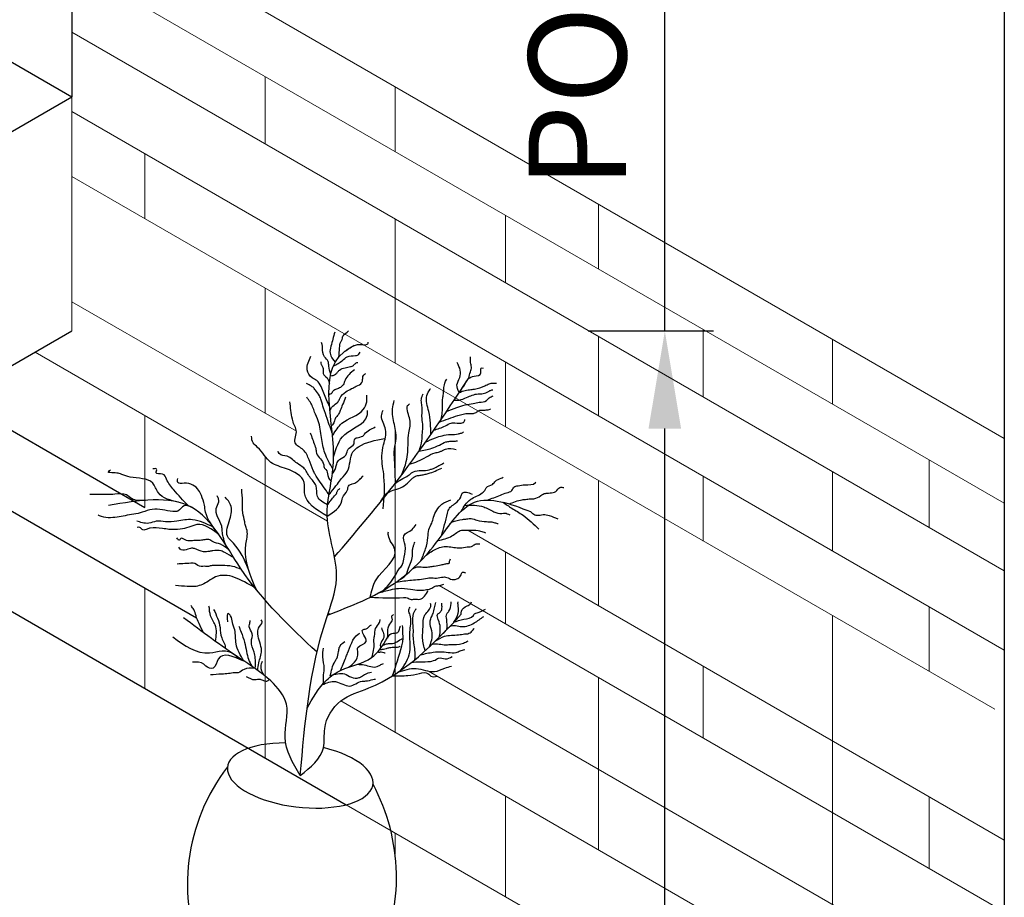
# Model space of a CAD drawing. Units: inches. Extents: x 5770 to 11891, y 3254 to 6808.
# Tile 10 of 15: x 6048 to 6073, y 3414 to 3436. Entities that reach past the tile are written whole.
import ezdxf

# ---------------------------------------------------------------- set-up
doc = ezdxf.new("R2010")
doc.units = ezdxf.units.IN
for name, color, linetype, lineweight in [('A-ANNO-DIMS', 2, 'Continuous', 18), ('A-DOOR', 4, 'Continuous', 25), ('A-FURN', 8, 'Continuous', 25), ('A-GLAZ', 4, 'Continuous', 25), ('A-WALL-PATT', 8, 'Continuous', 13)]:
    doc.layers.add(name, color=color, linetype=linetype, lineweight=lineweight)
doc.styles.get("Standard").update_dxf_attribs({"font": 'arial.ttf'})
doc.dimstyles.new('ISO-25', dxfattribs={"dimtxt": 2.5, "dimasz": 2.5, "dimexe": 1.25, "dimexo": 0.625, "dimtad": 1, "dimdec": 0, "dimlunit": 3, "dimtxsty": 'Standard', "dimcen": 2.5, "dimadec": 0, "dimazin": 0, "dimtfac": 1, "dimtdec": 0, "dimtmove": 0, "dimatfit": 3, "dimfxl": 1, "dimarcsym": 0})

# ---------------------------------------------------------------- blocks, each defined once
blk = doc.blocks.new('POT TREE')
for centre, radius, start, end in [((6057.241, 3414.341), 4.914, 142.3065, 203.4115), ((6052.61, 3414.509), 5.072, 334.4796, 28.1737), ((6055.12, 3416.4), 3.962, 226.5306, 307.3215), ((6054.997, 3414.987), 3.448, 228.9077, 309.4208)]:
    blk.add_arc(centre, radius, start, end)
blk.add_ellipse((6055.216, 3417.125), major_axis=(-1.864, 0.221), ratio=0.431649, start_param=4.964377, end_param=10.722247)
for points, knots in [([(6056.099, 3428.486), (6056.067, 3428.368), (6056.02, 3428.192), (6055.948, 3427.91), (6056.053, 3427.786), (6056.115, 3427.713)], [0, 0, 0, 0, 0.3734405, 0.5554394, 0.8239698, 0.8239698, 0.8239698, 0.8239698]), ([(6056.207, 3427.847), (6056.213, 3427.924), (6056.224, 3428.053), (6056.232, 3428.215), (6056.298, 3428.293), (6056.297, 3428.355), (6056.343, 3428.437), (6056.403, 3428.481), (6056.451, 3428.516)], [0, 0, 0, 0, 0.2339594, 0.3926456, 0.4649395, 0.5251746, 0.5691994, 0.7434006, 0.7434006, 0.7434006, 0.7434006]), ([(6055.216, 3417.125), (6055.336, 3418.48), (6055.487, 3420.181), (6056.331, 3422.342), (6055.715, 3423.715), (6056.354, 3425.55), (6055.582, 3427.539), (6056.504, 3428.093), (6056.597, 3428.149)], [0, 0, 0, 0, 4.080433, 5.124412, 6.755782, 8.14589, 10.974647, 11.292118, 11.292118, 11.292118, 11.292118]), ([(6056, 3427.411), (6055.979, 3427.477), (6055.946, 3427.582), (6055.946, 3427.752), (6055.806, 3427.869), (6055.784, 3428.034), (6055.784, 3428.159), (6055.766, 3428.202), (6055.759, 3428.218)], [0, 0, 0, 0, 0.2083526, 0.33199, 0.4828354, 0.7148467, 0.8018251, 0.8541407, 0.8541407, 0.8541407, 0.8541407]), ([(6056.371, 3428.002), (6056.422, 3428.039), (6056.532, 3428.118), (6056.727, 3428.199), (6056.886, 3428.139), (6056.964, 3428.199), (6056.961, 3428.223), (6056.96, 3428.232)], [0, 0, 0, 0, 0.1895566, 0.4093046, 0.6024508, 0.6414497, 0.6690189, 0.6690189, 0.6690189, 0.6690189]), ([(6055.967, 3426.585), (6055.915, 3426.698), (6055.838, 3426.866), (6055.755, 3427.096), (6055.662, 3427.248), (6055.479, 3427.316), (6055.344, 3427.566), (6055.436, 3427.759), (6055.492, 3427.874)], [0, 0, 0, 0, 0.371816, 0.552306, 0.74044, 0.877889, 1.120726, 1.482251, 1.482251, 1.482251, 1.482251]), ([(6056.064, 3427.611), (6056.145, 3427.655), (6056.269, 3427.724), (6056.427, 3427.889), (6056.588, 3427.869), (6056.72, 3427.903), (6056.741, 3427.953), (6056.749, 3427.972)], [0, 0, 0, 0, 0.2777951, 0.4294687, 0.6442569, 0.739735, 0.8005553, 0.8005553, 0.8005553, 0.8005553]), ([(6059.539, 3427.305), (6059.549, 3427.361), (6059.566, 3427.456), (6059.622, 3427.589), (6059.57, 3427.693), (6059.584, 3427.781), (6059.582, 3427.83), (6059.582, 3427.851)], [0, 0, 0, 0, 0.170284, 0.2915753, 0.4095788, 0.4920381, 0.5552227, 0.5552227, 0.5552227, 0.5552227]), ([(6055.746, 3427.727), (6055.745, 3427.704), (6055.742, 3427.656), (6055.802, 3427.595), (6055.813, 3427.51), (6055.793, 3427.397), (6055.923, 3427.324), (6055.949, 3427.228), (6055.963, 3427.179)], [0, 0, 0, 0, 0.0663677, 0.1385674, 0.2396579, 0.315315, 0.459478, 0.6088633, 0.6088633, 0.6088633, 0.6088633]), ([(6055.99, 3427.367), (6056.038, 3427.373), (6056.112, 3427.383), (6056.172, 3427.461), (6056.237, 3427.541), (6056.366, 3427.57), (6056.481, 3427.602), (6056.575, 3427.618), (6056.602, 3427.667), (6056.64, 3427.68), (6056.661, 3427.712), (6056.683, 3427.71), (6056.69, 3427.709)], [0, 0, 0, 0, 0.1365482, 0.2128619, 0.286554, 0.4402885, 0.5819688, 0.663825, 0.70336, 0.7384662, 0.7808805, 0.8013382, 0.8013382, 0.8013382, 0.8013382]), ([(6059.29, 3426.939), (6059.259, 3427.006), (6059.196, 3427.136), (6059.318, 3427.315), (6059.332, 3427.522), (6059.269, 3427.641), (6059.235, 3427.705)], [0, 0, 0, 0, 0.2050478, 0.4040971, 0.5914015, 0.8021175, 0.8021175, 0.8021175, 0.8021175]), ([(6059.29, 3426.939), (6059.343, 3427.011), (6059.426, 3427.125), (6059.515, 3427.313), (6059.674, 3427.364), (6059.891, 3427.379), (6059.816, 3427.58), (6059.884, 3427.567), (6059.904, 3427.563)], [0, 0, 0, 0, 0.2714027, 0.4305119, 0.5814667, 0.7785807, 0.9004742, 0.951926, 0.951926, 0.951926, 0.951926]), ([(6056.605, 3427.524), (6056.509, 3427.444), (6056.38, 3427.336), (6056.327, 3427.13), (6056.226, 3427.052), (6056.128, 3427.019), (6056.036, 3426.975), (6056.021, 3426.89), (6055.939, 3426.905), (6055.963, 3426.892), (6055.973, 3426.886)], [0, 0, 0, 0, 0.3596279, 0.4887998, 0.612961, 0.7210682, 0.8063572, 0.9000005, 0.9307269, 0.9560982, 0.9560982, 0.9560982, 0.9560982]), ([(6055.977, 3426.474), (6055.99, 3426.502), (6056.028, 3426.582), (6056.121, 3426.639), (6056.2, 3426.712), (6056.242, 3426.835), (6056.362, 3426.959), (6056.525, 3427.032), (6056.66, 3427.104), (6056.792, 3427.159), (6056.821, 3427.278), (6056.814, 3427.378), (6056.873, 3427.411), (6056.899, 3427.426)], [0, 0, 0, 0, 0.092214, 0.262657, 0.315664, 0.410651, 0.642816, 0.809137, 0.941877, 1.112577, 1.190652, 1.298465, 1.380948, 1.380948, 1.380948, 1.380948]), ([(6056.095, 3422.726), (6056.606, 3423.324), (6057.847, 3424.774), (6058.906, 3426.363), (6059.529, 3427.297)], [0, 0, 0, 0, 2.356363, 5.722003, 5.722003, 5.722003, 5.722003]), ([(6056.056, 3425.848), (6056.006, 3425.989), (6055.924, 3426.218), (6055.821, 3426.517), (6055.761, 3426.712), (6055.708, 3426.876), (6055.625, 3426.962), (6055.572, 3427.054), (6055.493, 3427.115), (6055.42, 3427.147), (6055.376, 3427.166)], [0, 0, 0, 0, 0.450624, 0.730149, 0.944944, 1.068285, 1.240151, 1.294175, 1.386296, 1.531529, 1.531529, 1.531529, 1.531529]), ([(6058.831, 3426.258), (6058.841, 3426.314), (6058.865, 3426.442), (6058.859, 3426.622), (6058.864, 3426.782), (6058.891, 3426.906), (6058.89, 3427.037), (6058.917, 3427.145), (6058.938, 3427.235), (6058.962, 3427.266), (6058.975, 3427.282)], [0, 0, 0, 0, 0.170516, 0.389854, 0.537702, 0.648645, 0.771235, 0.925907, 0.983276, 1.044113, 1.044113, 1.044113, 1.044113]), ([(6059.29, 3426.939), (6059.328, 3426.955), (6059.413, 3426.99), (6059.547, 3427.012), (6059.733, 3427.027), (6059.904, 3427.081), (6060.076, 3427.185), (6060.184, 3427.182), (6060.249, 3427.18)], [0, 0, 0, 0, 0.1235803, 0.275185, 0.4036544, 0.6827396, 0.8054315, 0.9964413, 0.9964413, 0.9964413, 0.9964413]), ([(6056.054, 3424.972), (6055.977, 3425.109), (6055.832, 3425.363), (6055.757, 3425.794), (6055.716, 3426.157), (6055.592, 3426.405), (6055.526, 3426.622), (6055.441, 3426.739), (6055.385, 3426.816)], [0, 0, 0, 0, 0.467532, 0.868461, 1.30425, 1.550258, 1.694478, 1.979135, 1.979135, 1.979135, 1.979135]), ([(6056.377, 3426.818), (6056.352, 3426.755), (6056.308, 3426.64), (6056.245, 3426.496), (6056.206, 3426.387), (6056.142, 3426.323), (6056.096, 3426.241), (6056.077, 3426.145), (6056.033, 3426.102), (6056.017, 3426.086)], [0, 0, 0, 0, 0.2037441, 0.3695408, 0.4757745, 0.5419956, 0.6389372, 0.7550592, 0.8219377, 0.8219377, 0.8219377, 0.8219377]), ([(6056.056, 3425.848), (6056.123, 3425.96), (6056.303, 3426.262), (6056.779, 3426.349), (6056.935, 3426.684), (6056.925, 3426.814), (6056.92, 3426.871)], [0, 0, 0, 0, 0.381595, 1.02877, 1.247836, 1.417617, 1.417617, 1.417617, 1.417617]), ([(6058.261, 3425.438), (6058.291, 3425.526), (6058.343, 3425.679), (6058.339, 3425.9), (6058.37, 3426.087), (6058.319, 3426.305), (6058.353, 3426.513), (6058.32, 3426.678), (6058.317, 3426.794), (6058.344, 3426.858), (6058.363, 3426.902)], [0, 0, 0, 0, 0.275722, 0.478551, 0.660336, 0.838715, 1.138147, 1.278337, 1.3416, 1.482993, 1.482993, 1.482993, 1.482993]), ([(6058.563, 3425.867), (6058.56, 3426.061), (6058.555, 3426.39), (6058.4, 3426.795), (6058.513, 3426.977), (6058.549, 3427.032), (6058.551, 3427.035)], [0, 0, 0, 0, 0.586596, 0.998805, 1.183674, 1.195699, 1.195699, 1.195699, 1.195699]), ([(6058.962, 3426.451), (6059.049, 3426.488), (6059.206, 3426.554), (6059.435, 3426.627), (6059.634, 3426.652), (6059.81, 3426.698), (6059.948, 3426.696), (6060.018, 3426.762), (6060.066, 3426.814), (6060.121, 3426.838), (6060.156, 3426.854)], [0, 0, 0, 0, 0.283693, 0.509561, 0.721223, 0.878225, 1.064501, 1.097071, 1.163997, 1.27537, 1.27537, 1.27537, 1.27537]), ([(6059.16, 3426.744), (6059.203, 3426.742), (6059.314, 3426.736), (6059.465, 3426.81), (6059.623, 3426.872), (6059.755, 3426.911), (6059.886, 3426.903), (6059.993, 3426.931), (6060.073, 3426.99), (6060.123, 3427.004), (6060.148, 3427.011)], [0, 0, 0, 0, 0.127889, 0.331448, 0.488133, 0.640962, 0.738356, 0.878783, 0.95994, 1.034357, 1.034357, 1.034357, 1.034357]), ([(6055.951, 3424.314), (6055.922, 3424.36), (6055.81, 3424.54), (6055.651, 3424.735), (6055.521, 3424.997), (6055.443, 3425.215), (6055.337, 3425.488), (6054.988, 3425.625), (6055.168, 3425.925), (6055.049, 3426.109), (6054.991, 3426.355), (6054.968, 3426.555), (6054.951, 3426.702)], [0, 0, 0, 0, 0.163711, 0.635891, 0.747378, 1.038356, 1.335228, 1.608013, 1.929766, 2.083186, 2.238732, 2.684923, 2.684923, 2.684923, 2.684923]), ([(6057.656, 3424.618), (6057.652, 3424.844), (6057.647, 3425.111), (6057.61, 3425.475), (6057.704, 3425.744), (6057.631, 3426.115), (6057.55, 3426.461), (6057.608, 3426.662), (6057.627, 3426.731)], [0, 0, 0, 0, 0.681083, 0.80233, 1.088716, 1.507668, 1.913958, 2.127718, 2.127718, 2.127718, 2.127718]), ([(6057.812, 3424.824), (6057.859, 3424.939), (6057.966, 3425.201), (6057.98, 3425.575), (6057.986, 3425.877), (6058.063, 3426.137), (6057.992, 3426.354), (6057.93, 3426.581), (6057.997, 3426.635), (6058.014, 3426.65)], [0, 0, 0, 0, 0.369909, 0.844557, 1.104784, 1.280935, 1.632037, 1.811788, 1.877667, 1.877667, 1.877667, 1.877667]), ([(6056.072, 3425.293), (6056.133, 3425.505), (6056.266, 3425.967), (6056.936, 3426.129), (6056.94, 3426.432), (6056.94, 3426.477)], [0, 0, 0, 0, 0.63578, 1.387331, 1.51754, 1.51754, 1.51754, 1.51754]), ([(6057.341, 3423.955), (6057.366, 3424.231), (6057.406, 3424.685), (6057.283, 3425.234), (6057.35, 3425.634), (6057.475, 3425.987), (6057.255, 3426.274), (6057.321, 3426.442), (6057.341, 3426.491)], [0, 0, 0, 0, 0.827857, 1.361014, 1.650618, 2.046768, 2.412651, 2.567148, 2.567148, 2.567148, 2.567148]), ([(6058.777, 3426.179), (6058.935, 3426.238), (6059.178, 3426.33), (6059.474, 3426.418), (6059.645, 3426.392), (6059.742, 3426.437), (6059.823, 3426.499), (6059.909, 3426.479), (6059.995, 3426.5), (6060.058, 3426.496), (6060.091, 3426.519), (6060.093, 3426.521)], [0, 0, 0, 0, 0.507912, 0.783706, 0.910821, 1.010253, 1.096153, 1.201661, 1.253677, 1.364003, 1.37374, 1.37374, 1.37374, 1.37374]), ([(6056.038, 3424.843), (6056.072, 3424.898), (6056.124, 3424.984), (6056.15, 3425.124), (6056.224, 3425.253), (6056.367, 3425.285), (6056.418, 3425.409), (6056.447, 3425.536), (6056.633, 3425.585), (6056.578, 3425.765), (6056.728, 3425.791), (6056.822, 3425.814), (6056.921, 3425.958), (6057.035, 3426.009), (6057.139, 3426.056)], [0, 0, 0, 0, 0.192002, 0.297038, 0.424323, 0.617299, 0.671515, 0.818658, 0.985168, 1.116162, 1.215874, 1.36714, 1.40004, 1.729093, 1.729093, 1.729093, 1.729093]), ([(6058.635, 3425.972), (6058.738, 3426.004), (6058.893, 3426.052), (6059.061, 3426.159), (6059.218, 3426.171), (6059.334, 3426.132), (6059.411, 3426.181), (6059.424, 3426.213), (6059.433, 3426.237), (6059.438, 3426.25)], [0, 0, 0, 0, 0.3205478, 0.4875046, 0.5825134, 0.7880727, 0.8113343, 0.8451959, 0.8888695, 0.8888695, 0.8888695, 0.8888695]), ([(6055.908, 3423.774), (6055.633, 3423.935), (6055.268, 3424.15), (6055.37, 3424.761), (6054.903, 3424.997), (6054.405, 3425.105), (6054.23, 3425.467), (6053.986, 3425.639), (6053.974, 3425.758), (6053.967, 3425.819)], [0, 0, 0, 0, 0.828493, 1.099501, 1.668133, 2.09953, 2.614238, 2.775429, 2.952527, 2.952527, 2.952527, 2.952527]), ([(6055.474, 3425.905), (6055.51, 3425.799), (6055.556, 3425.669), (6055.622, 3425.499), (6055.623, 3425.305), (6055.834, 3425.19), (6055.818, 3425.005), (6055.912, 3424.948), (6055.91, 3424.824), (6055.955, 3424.719), (6055.995, 3424.675), (6056.01, 3424.659)], [0, 0, 0, 0, 0.336378, 0.413394, 0.545538, 0.892702, 0.982578, 1.034981, 1.194475, 1.310114, 1.373927, 1.373927, 1.373927, 1.373927]), ([(6058.421, 3425.664), (6058.505, 3425.707), (6058.644, 3425.779), (6058.864, 3425.834), (6059.06, 3425.877), (6059.217, 3425.861), (6059.319, 3425.896), (6059.371, 3425.9), (6059.397, 3425.925), (6059.403, 3425.931)], [0, 0, 0, 0, 0.283751, 0.46616, 0.680012, 0.883292, 0.92268, 1.004792, 1.029716, 1.029716, 1.029716, 1.029716]), ([(6055.951, 3424.314), (6055.971, 3424.342), (6056.04, 3424.439), (6056.158, 3424.572), (6056.282, 3424.757), (6056.522, 3424.974), (6056.461, 3425.359), (6056.847, 3425.665), (6057.142, 3425.719), (6057.374, 3425.762)], [0, 0, 0, 0, 0.103537, 0.354957, 0.533042, 0.771117, 1.289622, 1.481323, 2.177692, 2.177692, 2.177692, 2.177692]), ([(6058.261, 3425.438), (6058.37, 3425.457), (6058.551, 3425.488), (6058.776, 3425.584), (6058.921, 3425.67), (6059.047, 3425.695), (6059.147, 3425.687), (6059.211, 3425.696), (6059.244, 3425.701)], [0, 0, 0, 0, 0.330364, 0.547312, 0.729955, 0.831797, 0.929171, 1.027126, 1.027126, 1.027126, 1.027126]), ([(6055.918, 3424.061), (6055.807, 3424.119), (6055.605, 3424.225), (6055.669, 3424.572), (6055.437, 3424.761), (6055.344, 3425.012), (6055.093, 3425.129), (6054.941, 3425.333), (6054.69, 3425.32), (6054.659, 3425.414), (6054.651, 3425.437)], [0, 0, 0, 0, 0.336493, 0.612709, 0.889575, 1.168065, 1.376144, 1.687858, 1.898629, 1.969205, 1.969205, 1.969205, 1.969205]), ([(6058.016, 3425.1), (6058.09, 3425.123), (6058.24, 3425.171), (6058.377, 3425.249), (6058.448, 3425.288)], [0, 0, 0, 0, 0.2298962, 0.4721725, 0.4721725, 0.4721725, 0.4721725]), ([(6058.448, 3425.288), (6058.521, 3425.33), (6058.626, 3425.39), (6058.771, 3425.413), (6058.839, 3425.441), (6058.89, 3425.468), (6059.001, 3425.522), (6059.117, 3425.5), (6059.209, 3425.483)], [0, 0, 0, 0, 0.2475713, 0.3610151, 0.4350864, 0.4658518, 0.5335827, 0.8019321, 0.8019321, 0.8019321, 0.8019321]), ([(6057.656, 3424.618), (6057.702, 3424.649), (6057.811, 3424.723), (6057.967, 3424.784), (6058.092, 3424.912), (6058.24, 3424.946), (6058.406, 3424.93), (6058.532, 3424.97), (6058.635, 3424.985), (6058.698, 3425.029), (6058.74, 3425.056), (6058.818, 3425.086), (6058.86, 3425.114), (6058.898, 3425.14)], [0, 0, 0, 0, 0.169056, 0.394003, 0.492513, 0.697087, 0.817485, 0.993544, 1.088828, 1.12295, 1.222592, 1.236685, 1.373008, 1.373008, 1.373008, 1.373008]), ([(6052.095, 3424.128), (6051.893, 3424.174), (6051.588, 3424.244), (6051.432, 3424.772), (6050.96, 3424.716), (6050.677, 3424.834), (6050.499, 3424.886), (6050.399, 3424.881), (6050.277, 3424.893), (6050.323, 3424.931), (6050.355, 3424.957)], [0, 0, 0, 0, 0.567769, 0.855404, 1.45352, 1.680633, 1.805502, 1.990259, 2.022667, 2.10403, 2.10403, 2.10403, 2.10403]), ([(6052.343, 3424.042), (6052.218, 3424.175), (6052.017, 3424.389), (6051.803, 3424.65), (6051.728, 3424.895), (6051.471, 3424.824), (6051.572, 3425.006), (6051.486, 3424.99), (6051.442, 3424.981)], [0, 0, 0, 0, 0.542059, 0.875538, 1.040909, 1.212562, 1.305796, 1.401779, 1.401779, 1.401779, 1.401779]), ([(6055.908, 3423.774), (6056.079, 3423.881), (6056.273, 3424.004), (6056.294, 3424.296), (6056.442, 3424.382), (6056.436, 3424.57), (6056.566, 3424.599), (6056.652, 3424.629), (6056.706, 3424.683), (6056.749, 3424.715), (6056.785, 3424.758), (6056.813, 3424.79), (6056.828, 3424.806)], [0, 0, 0, 0, 0.542154, 0.617715, 0.844166, 0.985871, 1.075503, 1.203366, 1.260039, 1.30062, 1.363236, 1.427954, 1.427954, 1.427954, 1.427954]), ([(6057.262, 3424.117), (6057.321, 3424.22), (6057.45, 3424.44), (6057.801, 3424.465), (6057.98, 3424.628), (6058.071, 3424.73), (6058.139, 3424.775), (6058.206, 3424.814), (6058.293, 3424.816), (6058.392, 3424.838), (6058.585, 3424.884), (6058.731, 3424.952), (6058.845, 3425.005)], [0, 0, 0, 0, 0.337635, 0.723781, 0.946218, 1.049759, 1.130989, 1.190526, 1.278087, 1.386469, 1.496256, 1.869563, 1.869563, 1.869563, 1.869563]), ([(6053.102, 3423.341), (6052.97, 3423.509), (6052.8, 3423.727), (6052.762, 3424.081), (6052.701, 3424.27), (6052.615, 3424.453), (6052.462, 3424.594), (6052.282, 3424.626), (6052.055, 3424.59), (6052.073, 3424.693), (6052.08, 3424.733)], [0, 0, 0, 0, 0.618637, 0.799298, 1.058478, 1.209073, 1.406969, 1.64005, 1.800082, 1.901705, 1.901705, 1.901705, 1.901705]), ([(6059.336, 3423.893), (6059.408, 3424.012), (6059.539, 3424.232), (6059.834, 3424.307), (6059.954, 3424.433), (6059.99, 3424.55), (6060.142, 3424.55), (6060.219, 3424.694), (6060.331, 3424.733), (6060.401, 3424.761), (6060.419, 3424.769)], [0, 0, 0, 0, 0.400751, 0.736445, 0.858272, 0.903351, 1.088652, 1.199604, 1.364928, 1.425221, 1.425221, 1.425221, 1.425221]), ([(6060.005, 3424.184), (6060.12, 3424.224), (6060.289, 3424.284), (6060.491, 3424.373), (6060.647, 3424.398), (6060.679, 3424.537), (6060.828, 3424.549), (6060.995, 3424.593), (6061.2, 3424.559), (6061.253, 3424.642), (6061.255, 3424.646)], [0, 0, 0, 0, 0.362377, 0.533627, 0.680662, 0.781131, 0.894461, 1.071848, 1.350792, 1.364242, 1.364242, 1.364242, 1.364242]), ([(6051.253, 3424.176), (6051.125, 3424.167), (6050.939, 3424.154), (6050.737, 3424.369), (6050.418, 3424.319), (6050.137, 3424.329), (6049.924, 3424.328), (6049.85, 3424.328), (6049.829, 3424.328)], [0, 0, 0, 0, 0.359068, 0.523067, 0.822385, 1.235556, 1.394449, 1.458006, 1.458006, 1.458006, 1.458006]), ([(6055.646, 3420.285), (6054.953, 3420.935), (6053.781, 3422.034), (6052.605, 3424.433), (6051.084, 3424.175), (6050.302, 3424.043)], [0, 0, 0, 0, 2.90941, 4.916012, 7.044236, 7.044236, 7.044236, 7.044236]), ([(6053.304, 3423.041), (6053.281, 3423.107), (6053.242, 3423.221), (6053.213, 3423.38), (6053.212, 3423.562), (6053.093, 3423.731), (6053.031, 3423.964), (6053.134, 3424.1), (6053.132, 3424.22), (6053.101, 3424.267), (6053.085, 3424.294)], [0, 0, 0, 0, 0.211774, 0.357994, 0.485633, 0.747154, 0.967772, 1.145664, 1.219006, 1.311906, 1.311906, 1.311906, 1.311906]), ([(6054.095, 3421.885), (6053.944, 3422.23), (6053.77, 3422.627), (6053.839, 3423.155), (6053.889, 3423.378), (6053.801, 3423.541), (6053.791, 3423.682), (6053.725, 3423.875), (6053.744, 3424.161), (6053.726, 3424.363), (6053.717, 3424.466)], [0, 0, 0, 0, 1.080878, 1.246414, 1.604364, 1.717568, 1.785951, 2.023042, 2.322993, 2.633061, 2.633061, 2.633061, 2.633061]), ([(6055.914, 3421.233), (6056.513, 3421.466), (6057.612, 3421.896), (6058.722, 3423.014), (6059.604, 3424.466), (6060.6, 3424.086), (6061.117, 3423.89)], [0, 0, 0, 0, 1.890611, 3.471497, 4.822432, 6.275175, 6.275175, 6.275175, 6.275175]), ([(6055.918, 3424.061), (6055.945, 3424.099), (6055.999, 3424.179), (6056.084, 3424.275), (6056.149, 3424.349), (6056.161, 3424.4), (6056.174, 3424.429), (6056.192, 3424.458), (6056.228, 3424.464), (6056.232, 3424.481), (6056.233, 3424.483)], [0, 0, 0, 0, 0.1386217, 0.290258, 0.3867591, 0.4253621, 0.4453978, 0.4816222, 0.5256508, 0.5320801, 0.5320801, 0.5320801, 0.5320801]), ([(6058.834, 3423.265), (6058.889, 3423.458), (6058.95, 3423.672), (6059.018, 3423.985), (6059.186, 3424.087), (6059.322, 3424.218), (6059.346, 3424.318), (6059.405, 3424.426), (6059.518, 3424.378), (6059.62, 3424.335)], [0, 0, 0, 0, 0.604353, 0.674045, 0.943845, 1.144991, 1.220534, 1.250613, 1.50171, 1.50171, 1.50171, 1.50171]), ([(6060.567, 3424.085), (6060.678, 3424.128), (6060.816, 3424.182), (6061.002, 3424.203), (6061.101, 3424.216), (6061.239, 3424.21), (6061.349, 3424.271), (6061.436, 3424.34), (6061.493, 3424.355), (6061.553, 3424.359), (6061.641, 3424.368), (6061.774, 3424.381), (6061.846, 3424.524), (6061.933, 3424.51), (6061.969, 3424.504)], [0, 0, 0, 0, 0.353763, 0.440342, 0.560317, 0.653707, 0.850793, 0.918069, 0.984218, 1.021734, 1.10046, 1.251722, 1.394315, 1.495093, 1.495093, 1.495093, 1.495093]), ([(6052.439, 3423.994), (6052.37, 3424.027), (6052.226, 3424.095), (6052.118, 3423.882), (6051.811, 3423.894), (6051.509, 3423.998), (6051.113, 3423.84), (6050.808, 3423.8), (6050.45, 3423.729), (6050.195, 3423.714), (6050.053, 3423.795), (6050.042, 3423.802)], [0, 0, 0, 0, 0.199212, 0.412008, 0.540446, 1.07049, 1.336159, 1.784437, 1.991377, 2.444385, 2.482266, 2.482266, 2.482266, 2.482266]), ([(6053.883, 3422.424), (6053.784, 3422.656), (6053.655, 3422.959), (6053.263, 3423.297), (6053.425, 3423.67), (6053.49, 3424.036), (6053.35, 3424.195), (6053.295, 3424.258)], [0, 0, 0, 0, 0.757434, 0.989726, 1.429851, 1.797091, 2.0391, 2.0391, 2.0391, 2.0391]), ([(6058.308, 3422.628), (6058.351, 3422.73), (6058.434, 3422.922), (6058.496, 3423.192), (6058.488, 3423.425), (6058.594, 3423.581), (6058.644, 3423.82), (6058.789, 3424.077), (6058.991, 3424.16), (6059.071, 3424.193)], [0, 0, 0, 0, 0.330054, 0.62708, 0.829768, 1.006692, 1.17071, 1.565043, 1.817324, 1.817324, 1.817324, 1.817324]), ([(6059.433, 3424.046), (6059.6, 3424.055), (6059.869, 3424.069), (6060.149, 3423.884), (6060.339, 3423.83), (6060.478, 3423.858), (6060.542, 3423.827), (6060.583, 3423.807)], [0, 0, 0, 0, 0.485239, 0.777831, 0.986173, 1.058443, 1.191294, 1.191294, 1.191294, 1.191294]), ([(6060.404, 3424.13), (6060.481, 3424.077), (6060.651, 3423.96), (6060.992, 3423.771), (6061.203, 3423.563), (6061.333, 3423.435)], [0, 0, 0, 0, 0.279864, 0.61954, 1.163685, 1.163685, 1.163685, 1.163685]), ([(6061.117, 3423.89), (6061.136, 3423.871), (6061.182, 3423.827), (6061.296, 3423.775), (6061.44, 3423.829), (6061.624, 3423.787), (6061.743, 3423.735), (6061.814, 3423.705)], [0, 0, 0, 0, 0.0805276, 0.1908805, 0.3539186, 0.511807, 0.7436297, 0.7436297, 0.7436297, 0.7436297]), ([(6052.99, 3423.487), (6052.815, 3423.575), (6052.516, 3423.724), (6052.091, 3423.65), (6051.784, 3423.611), (6051.538, 3423.669), (6051.349, 3423.573), (6051.175, 3423.596), (6051.077, 3423.631), (6051.031, 3423.647)], [0, 0, 0, 0, 0.568997, 0.970672, 1.257313, 1.499172, 1.696498, 1.862231, 2.008965, 2.008965, 2.008965, 2.008965]), ([(6053.128, 3423.304), (6052.945, 3423.442), (6052.696, 3423.63), (6052.359, 3423.482), (6052.123, 3423.424), (6051.892, 3423.426), (6051.639, 3423.459), (6051.442, 3423.491), (6051.286, 3423.441), (6051.178, 3423.384), (6051.122, 3423.496), (6051.062, 3423.486), (6051.038, 3423.481)], [0, 0, 0, 0, 0.612219, 0.830799, 1.053962, 1.343292, 1.51324, 1.82687, 1.906932, 2.021983, 2.121771, 2.190079, 2.190079, 2.190079, 2.190079]), ([(6057.366, 3421.886), (6057.481, 3422.012), (6057.623, 3422.17), (6057.727, 3422.4), (6057.798, 3422.472), (6057.863, 3422.574), (6057.878, 3422.763), (6057.949, 3422.994), (6057.791, 3423.308), (6058.079, 3423.393), (6058.156, 3423.515), (6058.186, 3423.561)], [0, 0, 0, 0, 0.507365, 0.630934, 0.750401, 0.807356, 0.99106, 1.298058, 1.54708, 1.813675, 1.980924, 1.980924, 1.980924, 1.980924]), ([(6059.095, 3423.618), (6059.188, 3423.647), (6059.316, 3423.688), (6059.486, 3423.699), (6059.611, 3423.72), (6059.774, 3423.648), (6059.944, 3423.627), (6060.099, 3423.632), (6060.195, 3423.604), (6060.255, 3423.589), (6060.284, 3423.582)], [0, 0, 0, 0, 0.290651, 0.399486, 0.511705, 0.662964, 0.915828, 1.024132, 1.123744, 1.212466, 1.212466, 1.212466, 1.212466]), ([(6057.012, 3421.697), (6057.043, 3421.847), (6057.134, 3422.295), (6057.798, 3422.701), (6057.549, 3423.097), (6057.468, 3423.242), (6057.473, 3423.338), (6057.475, 3423.369)], [0, 0, 0, 0, 0.465095, 1.381617, 1.582999, 1.778125, 1.868177, 1.868177, 1.868177, 1.868177]), ([(6058.747, 3423.147), (6058.871, 3423.174), (6059.088, 3423.221), (6059.303, 3423.434), (6059.548, 3423.398), (6059.734, 3423.43), (6059.881, 3423.375), (6059.944, 3423.354), (6059.967, 3423.347)], [0, 0, 0, 0, 0.377467, 0.661703, 0.822215, 1.087282, 1.215987, 1.286799, 1.286799, 1.286799, 1.286799]), ([(6053.386, 3422.911), (6053.319, 3422.965), (6053.196, 3423.066), (6052.997, 3423.089), (6052.887, 3423.18), (6052.784, 3423.172), (6052.672, 3423.146), (6052.482, 3423.153), (6052.305, 3423.116), (6052.168, 3423.234), (6052.112, 3423.113), (6052.076, 3423.184), (6052.058, 3423.22)], [0, 0, 0, 0, 0.2532, 0.467362, 0.579011, 0.658111, 0.76336, 0.926661, 1.225585, 1.285316, 1.367609, 1.455256, 1.455256, 1.455256, 1.455256]), ([(6057.782, 3422.159), (6057.848, 3422.194), (6057.948, 3422.247), (6057.983, 3422.484), (6058.115, 3422.666), (6058.083, 3422.874), (6058.11, 3422.976), (6058.129, 3423.052), (6058.148, 3423.095), (6058.156, 3423.114)], [0, 0, 0, 0, 0.206446, 0.312525, 0.690412, 0.832163, 0.923619, 1.005094, 1.065366, 1.065366, 1.065366, 1.065366]), ([(6058.442, 3422.774), (6058.529, 3422.832), (6058.661, 3422.92), (6058.919, 3423.02), (6059.139, 3422.965), (6059.366, 3422.954), (6059.496, 3422.989), (6059.612, 3422.989), (6059.663, 3423.038), (6059.737, 3423.066), (6059.786, 3423.066), (6059.817, 3423.066)], [0, 0, 0, 0, 0.314833, 0.47653, 0.809502, 0.966328, 1.154795, 1.214977, 1.302026, 1.35401, 1.447623, 1.447623, 1.447623, 1.447623]), ([(6053.514, 3422.708), (6053.439, 3422.751), (6053.333, 3422.813), (6053.158, 3422.904), (6053.015, 3422.892), (6052.87, 3422.865), (6052.704, 3422.836), (6052.574, 3422.924), (6052.436, 3422.96), (6052.327, 3422.917), (6052.207, 3422.881), (6052.131, 3422.931), (6052.115, 3422.96), (6052.105, 3422.978)], [0, 0, 0, 0, 0.261711, 0.370131, 0.582712, 0.66806, 0.81934, 1.066406, 1.111973, 1.240926, 1.409664, 1.445312, 1.505627, 1.505627, 1.505627, 1.505627]), ([(6053.711, 3422.403), (6053.634, 3422.436), (6053.477, 3422.502), (6053.266, 3422.504), (6053.133, 3422.505), (6053.046, 3422.504), (6052.964, 3422.514), (6052.871, 3422.48), (6052.791, 3422.486), (6052.715, 3422.486), (6052.602, 3422.477), (6052.532, 3422.566), (6052.333, 3422.563), (6052.195, 3422.552), (6052.061, 3422.542)], [0, 0, 0, 0, 0.248192, 0.507613, 0.621751, 0.648397, 0.770142, 0.863413, 0.939511, 1.008, 1.091792, 1.268763, 1.280175, 1.684599, 1.684599, 1.684599, 1.684599]), ([(6058.106, 3422.43), (6058.148, 3422.451), (6058.241, 3422.497), (6058.39, 3422.448), (6058.529, 3422.477), (6058.674, 3422.492), (6058.804, 3422.517), (6058.927, 3422.547), (6058.989, 3422.56), (6059.04, 3422.564), (6059.031, 3422.619), (6059.053, 3422.65), (6059.07, 3422.674)], [0, 0, 0, 0, 0.136191, 0.301111, 0.440041, 0.556702, 0.739007, 0.8386, 0.929419, 0.944819, 0.971199, 1.059876, 1.059876, 1.059876, 1.059876]), ([(6054.055, 3421.936), (6053.704, 3422.141), (6053.282, 3422.388), (6052.829, 3422.079), (6052.591, 3421.952), (6052.296, 3421.974), (6052.122, 3421.985), (6052.023, 3421.991)], [0, 0, 0, 0, 1.043584, 1.256005, 1.602855, 1.825433, 2.126041, 2.126041, 2.126041, 2.126041]), ([(6057.679, 3422.086), (6057.809, 3422.103), (6058.076, 3422.14), (6058.365, 3422.152), (6058.546, 3422.197), (6058.621, 3422.188), (6058.735, 3422.179), (6058.839, 3422.21), (6058.968, 3422.217), (6059.07, 3422.14), (6059.222, 3422.147), (6059.333, 3422.22), (6059.355, 3422.359), (6059.421, 3422.328), (6059.447, 3422.316)], [0, 0, 0, 0, 0.393084, 0.806547, 0.867321, 0.945801, 1.031735, 1.209105, 1.268822, 1.409537, 1.566345, 1.691075, 1.797982, 1.871323, 1.871323, 1.871323, 1.871323]), ([(6057.214, 3421.8), (6057.318, 3421.831), (6057.489, 3421.882), (6057.767, 3421.934), (6058.014, 3421.911), (6058.239, 3421.862), (6058.413, 3421.88), (6058.536, 3421.902), (6058.624, 3421.948), (6058.698, 3421.994), (6058.799, 3421.986), (6058.862, 3422.016), (6058.895, 3422.032)], [0, 0, 0, 0, 0.325945, 0.533976, 0.844352, 1.062897, 1.220077, 1.365852, 1.432613, 1.519427, 1.617117, 1.724591, 1.724591, 1.724591, 1.724591]), ([(6057.012, 3421.697), (6057.294, 3421.68), (6057.596, 3421.661), (6057.945, 3421.695), (6058.029, 3421.623), (6058.155, 3421.652), (6058.353, 3421.615), (6058.438, 3421.764), (6058.496, 3421.868)], [0, 0, 0, 0, 0.853157, 0.913238, 1.027604, 1.147747, 1.282906, 1.590947, 1.590947, 1.590947, 1.590947]), ([(6058.416, 3420.323), (6058.386, 3420.43), (6058.328, 3420.635), (6058.378, 3420.941), (6058.35, 3421.253), (6058.588, 3421.407), (6058.557, 3421.519), (6058.552, 3421.536)], [0, 0, 0, 0, 0.328571, 0.626938, 0.928595, 1.215628, 1.267031, 1.267031, 1.267031, 1.267031]), ([(6058.53, 3420.428), (6058.572, 3420.547), (6058.639, 3420.74), (6058.526, 3420.984), (6058.558, 3421.16), (6058.632, 3421.286), (6058.65, 3421.419), (6058.678, 3421.511), (6058.692, 3421.555)], [0, 0, 0, 0, 0.358902, 0.587337, 0.76495, 0.869476, 1.023512, 1.159883, 1.159883, 1.159883, 1.159883]), ([(6058.778, 3420.669), (6058.794, 3420.753), (6058.823, 3420.909), (6058.77, 3421.086), (6058.703, 3421.247), (6058.802, 3421.3), (6058.856, 3421.388), (6058.849, 3421.477), (6058.842, 3421.531), (6058.841, 3421.54)], [0, 0, 0, 0, 0.2483439, 0.4590321, 0.5916982, 0.6641726, 0.7593593, 0.8908118, 0.9202375, 0.9202375, 0.9202375, 0.9202375]), ([(6058.975, 3420.87), (6058.978, 3420.953), (6058.984, 3421.082), (6058.943, 3421.261), (6059.065, 3421.361), (6059.083, 3421.483), (6059.082, 3421.566), (6059.082, 3421.58)], [0, 0, 0, 0, 0.2582523, 0.3969468, 0.4904461, 0.695008, 0.7388085, 0.7388085, 0.7388085, 0.7388085]), ([(6059.152, 3421.054), (6059.201, 3421.128), (6059.284, 3421.251), (6059.266, 3421.418), (6059.263, 3421.506), (6059.255, 3421.546), (6059.26, 3421.568), (6059.261, 3421.577)], [0, 0, 0, 0, 0.257058, 0.428605, 0.4834756, 0.5237874, 0.549599, 0.549599, 0.549599, 0.549599]), ([(6059.343, 3421.256), (6059.341, 3421.284), (6059.335, 3421.38), (6059.457, 3421.47), (6059.583, 3421.506), (6059.601, 3421.56), (6059.608, 3421.58)], [0, 0, 0, 0, 0.0794153, 0.2808618, 0.3854818, 0.4459081, 0.4459081, 0.4459081, 0.4459081]), ([(6052.739, 3420.786), (6052.7, 3420.865), (6052.63, 3421.006), (6052.541, 3421.199), (6052.517, 3421.351), (6052.45, 3421.424), (6052.432, 3421.46), (6052.424, 3421.478)], [0, 0, 0, 0, 0.2642834, 0.4700989, 0.6421411, 0.7030564, 0.762993, 0.762993, 0.762993, 0.762993]), ([(6053.044, 3420.562), (6053.066, 3420.709), (6053.095, 3420.908), (6052.951, 3421.137), (6052.889, 3421.29), (6052.893, 3421.412), (6052.878, 3421.454), (6052.875, 3421.462)], [0, 0, 0, 0, 0.4211546, 0.57187, 0.7991017, 0.9053512, 0.9310241, 0.9310241, 0.9310241, 0.9310241]), ([(6052.998, 3421.383), (6053.069, 3421.231), (6053.178, 3420.996), (6053.167, 3420.646), (6053.315, 3420.473), (6053.292, 3420.385)], [0, 0, 0, 0, 0.491062, 0.760416, 1.043151, 1.043151, 1.043151, 1.043151]), ([(6053.773, 3420.059), (6053.687, 3420.202), (6053.539, 3420.45), (6053.57, 3420.809), (6053.47, 3421.04), (6053.464, 3421.185), (6053.334, 3421.344), (6053.345, 3421.18), (6053.354, 3421.06)], [0, 0, 0, 0, 0.486789, 0.841844, 1.040934, 1.218264, 1.298858, 1.518651, 1.518651, 1.518651, 1.518651]), ([(6055.216, 3417.125), (6055.482, 3417.339), (6055.887, 3417.665), (6055.786, 3418.448), (6056.191, 3419.123), (6057.73, 3419.549), (6058.63, 3420.501), (6059.343, 3421.256)], [0, 0, 0, 0, 0.930345, 1.419949, 2.238038, 3.028538, 6.05988, 6.05988, 6.05988, 6.05988]), ([(6057.456, 3420.669), (6057.458, 3420.714), (6057.461, 3420.828), (6057.468, 3420.993), (6057.61, 3421.098), (6057.54, 3421.196), (6057.581, 3421.234), (6057.602, 3421.252)], [0, 0, 0, 0, 0.1343407, 0.3452256, 0.4766174, 0.5519158, 0.6245951, 0.6245951, 0.6245951, 0.6245951]), ([(6057.797, 3419.822), (6057.895, 3419.97), (6058.058, 3420.217), (6058.023, 3420.591), (6058.021, 3420.906), (6058.085, 3421.155), (6057.983, 3421.342), (6058.015, 3421.409), (6058.029, 3421.438)], [0, 0, 0, 0, 0.513113, 0.856104, 1.090795, 1.466282, 1.586294, 1.677635, 1.677635, 1.677635, 1.677635]), ([(6058.154, 3420.095), (6058.158, 3420.159), (6058.172, 3420.346), (6058.103, 3420.595), (6058.127, 3420.94), (6058.062, 3421.219), (6058.171, 3421.378), (6058.187, 3421.402)], [0, 0, 0, 0, 0.19319, 0.561329, 0.753109, 1.237908, 1.324083, 1.324083, 1.324083, 1.324083]), ([(6059.152, 3421.054), (6059.233, 3421.084), (6059.395, 3421.143), (6059.621, 3421.157), (6059.682, 3421.28), (6059.806, 3421.307), (6059.894, 3421.354), (6059.962, 3421.391)], [0, 0, 0, 0, 0.267226, 0.5296906, 0.5844534, 0.6515853, 0.8870376, 0.8870376, 0.8870376, 0.8870376]), ([(6055.216, 3417.125), (6055.028, 3417.441), (6054.69, 3418.011), (6055.01, 3418.94), (6054.413, 3419.655), (6053.442, 3420.255), (6052.702, 3420.811), (6052.226, 3421.169)], [0, 0, 0, 0, 1.055483, 1.900743, 2.620176, 3.60344, 5.381171, 5.381171, 5.381171, 5.381171]), ([(6054.061, 3419.866), (6054.068, 3419.957), (6054.079, 3420.1), (6054.028, 3420.331), (6053.923, 3420.531), (6054.033, 3420.764), (6053.883, 3420.907), (6053.928, 3421.027), (6053.93, 3421.08), (6053.931, 3421.096)], [0, 0, 0, 0, 0.272035, 0.425717, 0.710261, 0.906634, 1.101207, 1.212004, 1.260886, 1.260886, 1.260886, 1.260886]), ([(6054.127, 3419.819), (6054.134, 3419.883), (6054.151, 3420.055), (6054.284, 3420.366), (6054.128, 3420.634), (6054.128, 3420.83), (6054.146, 3420.941), (6054.272, 3421.023), (6054.226, 3421.098), (6054.215, 3421.116)], [0, 0, 0, 0, 0.195211, 0.519287, 0.955652, 1.032782, 1.103683, 1.291016, 1.349146, 1.349146, 1.349146, 1.349146]), ([(6057.053, 3420.154), (6057.087, 3420.273), (6057.127, 3420.416), (6057.094, 3420.599), (6057.134, 3420.723), (6057.112, 3420.9), (6057.249, 3421.009), (6057.261, 3421.099), (6057.265, 3421.127)], [0, 0, 0, 0, 0.363375, 0.43631, 0.549947, 0.745445, 0.929842, 1.013173, 1.013173, 1.013173, 1.013173]), ([(6058.879, 3420.771), (6058.911, 3420.802), (6058.969, 3420.858), (6059.087, 3421.017), (6059.377, 3420.897), (6059.673, 3421.018), (6059.84, 3421.144), (6059.919, 3421.204)], [0, 0, 0, 0, 0.137624, 0.244175, 0.554938, 0.881931, 1.180494, 1.180494, 1.180494, 1.180494]), ([(6053.642, 3420.954), (6053.662, 3420.902), (6053.715, 3420.767), (6053.793, 3420.552), (6053.835, 3420.316), (6053.882, 3420.103), (6053.945, 3419.983), (6053.976, 3419.924)], [0, 0, 0, 0, 0.165675, 0.436943, 0.682575, 0.886472, 1.08622, 1.08622, 1.08622, 1.08622]), ([(6056.247, 3419.816), (6056.291, 3419.926), (6056.35, 3420.074), (6056.485, 3420.39), (6056.556, 3420.656), (6056.729, 3420.766), (6056.742, 3420.774)], [0, 0, 0, 0, 0.35488, 0.476802, 1.039524, 1.08736, 1.08736, 1.08736, 1.08736]), ([(6056.452, 3419.898), (6056.508, 3419.938), (6056.636, 3420.029), (6056.717, 3420.226), (6056.651, 3420.472), (6057.08, 3420.5), (6056.699, 3420.872), (6056.935, 3420.872), (6056.98, 3420.957), (6057.032, 3420.98), (6057.044, 3420.985)], [0, 0, 0, 0, 0.204713, 0.46444, 0.597521, 0.857548, 1.172597, 1.267469, 1.399027, 1.436243, 1.436243, 1.436243, 1.436243]), ([(6057.295, 3420.91), (6057.339, 3420.813), (6057.386, 3420.706), (6057.31, 3420.569), (6057.247, 3420.492), (6057.272, 3420.415), (6057.279, 3420.391)], [0, 0, 0, 0, 0.2830174, 0.3089283, 0.4692506, 0.5421239, 0.5421239, 0.5421239, 0.5421239]), ([(6057.447, 3420.644), (6057.472, 3420.689), (6057.522, 3420.778), (6057.639, 3420.773), (6057.737, 3420.788), (6057.748, 3420.871), (6057.774, 3420.921), (6057.782, 3420.946), (6057.784, 3420.951)], [0, 0, 0, 0, 0.1422118, 0.2807161, 0.3239465, 0.4223122, 0.482263, 0.4998664, 0.4998664, 0.4998664, 0.4998664]), ([(6057.584, 3419.681), (6057.668, 3419.936), (6057.765, 3420.233), (6057.858, 3420.59), (6057.847, 3420.766), (6057.843, 3420.897), (6057.84, 3420.973)], [0, 0, 0, 0, 0.806681, 0.937437, 1.101821, 1.330318, 1.330318, 1.330318, 1.330318]), ([(6058.673, 3420.565), (6058.75, 3420.617), (6058.93, 3420.739), (6059.207, 3420.71), (6059.403, 3420.756), (6059.525, 3420.753), (6059.619, 3420.812), (6059.659, 3420.875), (6059.677, 3420.904)], [0, 0, 0, 0, 0.271953, 0.635002, 0.791848, 0.875249, 0.996666, 1.099954, 1.099954, 1.099954, 1.099954]), ([(6051.951, 3420.679), (6052.253, 3420.458), (6052.744, 3420.099), (6053.387, 3420.431), (6053.629, 3420.113), (6053.661, 3420.133)], [0, 0, 0, 0, 1.030033, 1.673917, 1.823017, 1.823017, 1.823017, 1.823017]), ([(6055.392, 3418.845), (6055.534, 3419.106), (6055.75, 3419.504), (6056.36, 3419.92), (6057.053, 3420.019), (6057.328, 3420.456), (6057.447, 3420.644)], [0, 0, 0, 0, 0.875687, 1.330988, 2.175672, 2.81649, 2.81649, 2.81649, 2.81649]), ([(6055.986, 3419.68), (6056.013, 3419.808), (6056.047, 3419.967), (6056.172, 3420.15), (6056.197, 3420.276), (6056.208, 3420.388), (6056.256, 3420.483), (6056.314, 3420.526), (6056.357, 3420.559)], [0, 0, 0, 0, 0.3869465, 0.4790906, 0.6576508, 0.7623461, 0.814256, 0.9738073, 0.9738073, 0.9738073, 0.9738073]), ([(6057.323, 3420.452), (6057.349, 3420.468), (6057.406, 3420.502), (6057.523, 3420.509), (6057.673, 3420.511), (6057.758, 3420.617), (6057.826, 3420.626), (6057.835, 3420.627)], [0, 0, 0, 0, 0.0918133, 0.1957838, 0.3452755, 0.5238583, 0.5506495, 0.5506495, 0.5506495, 0.5506495]), ([(6057.456, 3420.669), (6057.456, 3420.664), (6057.457, 3420.655), (6057.45, 3420.648), (6057.448, 3420.644), (6057.447, 3420.643), (6057.446, 3420.643)], [0, 0, 0, 0, 0.01534388, 0.02460385, 0.02767794, 0.0287637, 0.0287637, 0.0287637, 0.0287637]), ([(6058.53, 3420.428), (6058.544, 3420.444), (6058.637, 3420.542), (6058.856, 3420.462), (6059.111, 3420.49), (6059.319, 3420.469), (6059.457, 3420.55), (6059.51, 3420.571), (6059.522, 3420.575)], [0, 0, 0, 0, 0.061886, 0.394711, 0.553699, 0.854621, 0.985558, 1.024465, 1.024465, 1.024465, 1.024465]), ([(6053.773, 3420.059), (6053.5, 3420.177), (6053.116, 3420.344), (6053.043, 3419.816), (6052.819, 3419.898), (6052.698, 3420.039), (6052.564, 3420.035), (6052.455, 3420.032)], [0, 0, 0, 0, 0.656939, 0.924352, 1.118511, 1.190349, 1.483547, 1.483547, 1.483547, 1.483547]), ([(6055.803, 3420.39), (6055.791, 3420.316), (6055.763, 3420.14), (6055.847, 3419.894), (6055.792, 3419.663), (6055.807, 3419.527), (6055.793, 3419.467), (6055.793, 3419.465)], [0, 0, 0, 0, 0.2230459, 0.5273899, 0.747132, 0.9216994, 0.9298862, 0.9298862, 0.9298862, 0.9298862]), ([(6057.199, 3420.291), (6057.212, 3420.29), (6057.235, 3420.289), (6057.266, 3420.29), (6057.305, 3420.304), (6057.345, 3420.275), (6057.38, 3420.272), (6057.392, 3420.271)], [0, 0, 0, 0, 0.0402932, 0.0686689, 0.0924745, 0.159771, 0.197884, 0.197884, 0.197884, 0.197884]), ([(6057.253, 3420.356), (6057.286, 3420.358), (6057.344, 3420.36), (6057.428, 3420.385), (6057.521, 3420.414), (6057.618, 3420.41), (6057.71, 3420.413), (6057.756, 3420.429), (6057.779, 3420.438)], [0, 0, 0, 0, 0.0996796, 0.1729656, 0.2621178, 0.3889537, 0.4629495, 0.535647, 0.535647, 0.535647, 0.535647]), ([(6058.301, 3420.22), (6058.409, 3420.246), (6058.59, 3420.289), (6058.91, 3420.312), (6059.158, 3420.238), (6059.333, 3420.334), (6059.392, 3420.347), (6059.432, 3420.355)], [0, 0, 0, 0, 0.331341, 0.555581, 0.967429, 1.027217, 1.147289, 1.147289, 1.147289, 1.147289]), ([(6054.242, 3420.05), (6054.224, 3420.007), (6054.174, 3419.889), (6054.24, 3419.774), (6054.282, 3419.701)], [0, 0, 0, 0, 0.1342896, 0.3683703, 0.3683703, 0.3683703, 0.3683703]), ([(6056.685, 3419.976), (6056.741, 3419.974), (6056.908, 3419.968), (6057.117, 3419.863), (6057.266, 3419.961), (6057.321, 3419.985), (6057.352, 3419.998)], [0, 0, 0, 0, 0.1685942, 0.5092383, 0.5884198, 0.6891895, 0.6891895, 0.6891895, 0.6891895]), ([(6058.067, 3420.024), (6058.14, 3420.032), (6058.301, 3420.047), (6058.519, 3420.035), (6058.679, 3420.081), (6058.791, 3420.165), (6058.941, 3420.084), (6059.05, 3420.144), (6059.106, 3420.174)], [0, 0, 0, 0, 0.220029, 0.483981, 0.651902, 0.710145, 0.884481, 1.067265, 1.067265, 1.067265, 1.067265]), ([(6054.061, 3419.866), (6053.96, 3419.879), (6053.8, 3419.899), (6053.658, 3419.744), (6053.512, 3419.77), (6053.375, 3419.727), (6053.167, 3419.725), (6053.012, 3419.712), (6052.914, 3419.704)], [0, 0, 0, 0, 0.285648, 0.454923, 0.552406, 0.70467, 0.879767, 1.172939, 1.172939, 1.172939, 1.172939]), ([(6055.986, 3419.68), (6056.112, 3419.723), (6056.306, 3419.789), (6056.518, 3419.627), (6056.688, 3419.609), (6056.801, 3419.671), (6056.896, 3419.74), (6056.987, 3419.761), (6057.041, 3419.773)], [0, 0, 0, 0, 0.366542, 0.563229, 0.761998, 0.833943, 0.94708, 1.109952, 1.109952, 1.109952, 1.109952]), ([(6057.584, 3419.681), (6057.717, 3419.68), (6057.952, 3419.677), (6058.234, 3419.727), (6058.471, 3419.79), (6058.571, 3419.636), (6058.667, 3419.66), (6058.727, 3419.675)], [0, 0, 0, 0, 0.391291, 0.69538, 0.908511, 1.010802, 1.173393, 1.173393, 1.173393, 1.173393]), ([(6057.721, 3419.77), (6057.876, 3419.825), (6058.184, 3419.934), (6058.595, 3419.73), (6058.889, 3419.868), (6059.034, 3419.914), (6059.092, 3419.932)], [0, 0, 0, 0, 0.477597, 0.949756, 1.226232, 1.409018, 1.409018, 1.409018, 1.409018]), ([(6053.83, 3419.664), (6053.902, 3419.623), (6054.015, 3419.558), (6054.161, 3419.609), (6054.246, 3419.57), (6054.303, 3419.551), (6054.374, 3419.54), (6054.402, 3419.569), (6054.418, 3419.587)], [0, 0, 0, 0, 0.2367663, 0.3700356, 0.4202495, 0.5125068, 0.5554594, 0.6234894, 0.6234894, 0.6234894, 0.6234894]), ([(6055.777, 3419.452), (6055.893, 3419.502), (6056.131, 3419.605), (6056.478, 3419.319), (6056.718, 3419.552), (6056.928, 3419.543), (6057.04, 3419.582), (6057.125, 3419.593), (6057.148, 3419.596)], [0, 0, 0, 0, 0.355506, 0.732116, 1.076752, 1.168114, 1.354305, 1.424852, 1.424852, 1.424852, 1.424852])]:
    blk.add_open_spline(points, degree=3, knots=knots)
blk.add_open_spline([(6058.959, 3423.437), (6059.013, 3423.509), (6059.068, 3423.581), (6059.123, 3423.654)], degree=3)
blk = doc.blocks.new('*D38')
at = {"layer": 'A-ANNO-DIMS', "color": 0, "lineweight": -2, "transparency": 16777216}
for p, q in [((6064.558, 3428.516), (6064.558, 3471.974)), ((6062.594, 3428.516), (6065.808, 3428.516)), ((6064.558, 3413.754), (6064.558, 3426.016)), ((6062.594, 3411.254), (6065.808, 3411.254))]:
    blk.add_line(p, q, dxfattribs=at)
at = {"layer": 'A-ANNO-DIMS', "color": 0, "transparency": 16777216}
for points in [[(6064.141, 3426.016), (6064.975, 3426.016), (6064.558, 3428.516)], [(6064.141, 3413.754), (6064.975, 3413.754), (6064.558, 3411.254)]]:
    blk.add_solid(points, dxfattribs=at)
at = {"layer": 'Defpoints', "color": 0, "transparency": 16777216}
for p in [(6061.969, 3428.516), (6064.558, 3428.516), (6061.969, 3411.254)]:
    blk.add_point(p, dxfattribs=at)
at = {"layer": 'A-ANNO-DIMS', "color": 0, "transparency": 16777216, "insert": (6062.64, 3451.495), "char_height": 2.5, "attachment_point": 5, "rotation": 90}
blk.add_mtext('POTTED PLANT 1\'-5 1/2"', dxfattribs=at)

msp = doc.modelspace()

# ---------------------------------------------------------------- linework, layer by layer
at = {"layer": 'A-DOOR'}
msp.add_line((6073.257, 3462.723), (6073.257, 3386.42), dxfattribs=at)
at = {"layer": 'A-FURN'}
for p, q in [((6049.365, 3476.517), (6049.365, 3434.517)), ((5975.971, 3462.811), (6056.394, 3416.379)), ((6044.169, 3431.517), (6049.365, 3434.517)), ((6044.169, 3425.517), (6049.365, 3428.517)), ((6046.383, 3426.796), (6051.234, 3423.996)), ((6044.597, 3425.765), (6052.561, 3421.167))]:
    msp.add_line(p, q, dxfattribs=at)
at = {"layer": 'A-GLAZ'}
msp.add_line((6007.795, 3458.517), (6049.365, 3434.517), dxfattribs=at)
at = {"layer": 'A-WALL-PATT'}
for p, q in [((6049.365, 3439.555), (6073.257, 3425.761)), ((6049.365, 3437.894), (6073.257, 3424.1)), ((6049.365, 3436.168), (6073.257, 3422.374)), ((6054.319, 3435.033), (6054.319, 3433.308)), ((6057.645, 3434.775), (6057.645, 3433.113)), ((6049.365, 3434.517), (6049.365, 3428.517)), ((6049.365, 3434.136), (6073.257, 3420.342)), ((6051.234, 3433.057), (6051.234, 3431.396)), ((6049.365, 3432.475), (6073.011, 3418.823)), ((6062.859, 3431.764), (6062.859, 3430.103)), ((6057.645, 3431.388), (6057.645, 3427.694)), ((6060.48, 3431.477), (6060.48, 3429.751)), ((6054.319, 3429.614), (6054.319, 3426.406)), ((6049.365, 3429.266), (6055.117, 3425.945)), ((6062.859, 3428.377), (6062.859, 3426.345)), ((6065.543, 3428.553), (6065.543, 3426.828)), ((6068.858, 3428.301), (6068.858, 3426.639)), ((6048.421, 3427.972), (6055.917, 3423.644)), ((6060.48, 3427.719), (6060.48, 3426.058)), ((6051.234, 3426.348), (6051.234, 3423.996)), ((6057.645, 3426.035), (6057.645, 3418.232)), ((6054.319, 3425.302), (6054.319, 3417.577)), ((6071.332, 3425.211), (6071.332, 3423.486)), ((6065.543, 3424.795), (6065.543, 3423.134)), ((6068.858, 3424.914), (6068.858, 3422.882)), ((6062.859, 3424.684), (6062.859, 3421.475)), ((6060.48, 3424.11), (6060.48, 3424.078)), ((6059.111, 3423.639), (6059.13, 3423.629)), ((6059.508, 3423.41), (6073.257, 3415.472)), ((6060.48, 3422.849), (6060.48, 3421.01)), ((6051.234, 3421.934), (6051.234, 3419.358)), ((6058.778, 3421.992), (6073.257, 3413.633)), ((6055.931, 3421.284), (6055.977, 3421.257)), ((6071.332, 3421.453), (6071.332, 3419.792)), ((6068.858, 3421.22), (6068.858, 3411.758)), ((6057.336, 3420.472), (6057.347, 3420.466)), ((6058.086, 3420.04), (6058.106, 3420.028)), ((6058.499, 3419.801), (6072.818, 3411.534)), ((6065.543, 3419.925), (6065.543, 3418.086)), ((6062.859, 3419.636), (6062.859, 3415.222)), ((6056.253, 3419.036), (6071.032, 3410.503)), ((6060.48, 3416.595), (6060.48, 3414.02)), ((6071.332, 3416.584), (6071.332, 3414.744)), ((6056.394, 3416.379), (6068.801, 3409.216)), ((6057.645, 3415.657), (6057.645, 3415.116))]:
    msp.add_line(p, q, dxfattribs=at)

# ---------------------------------------------------------------- block references
at = {"layer": 'A-FURN'}
msp.add_blockref('POT TREE', (0, 0), dxfattribs=at)

# ---------------------------------------------------------------- dimensions: what is measured, and where the dimension line sits
at = {"layer": 'A-ANNO-DIMS'}
dim = msp.add_linear_dim(base=(6064.558, 3428.516), p1=(6061.969, 3411.254), p2=(6061.969, 3428.516), angle=90, text='POTTED PLANT <>', dimstyle='ISO-25', override={"dimdec": 1, "dimlfac": 1, "dimrnd": 0, "dimzin": 1, "dimdsep": 46, "dimlunit": 4, "dimfrac": 2}, dxfattribs=at)
dim.commit()
dim.dimension.update_dxf_attribs({"geometry": '*D38', "text_midpoint": (6062.64, 3451.495)})

doc.saveas('drawing.dxf')
